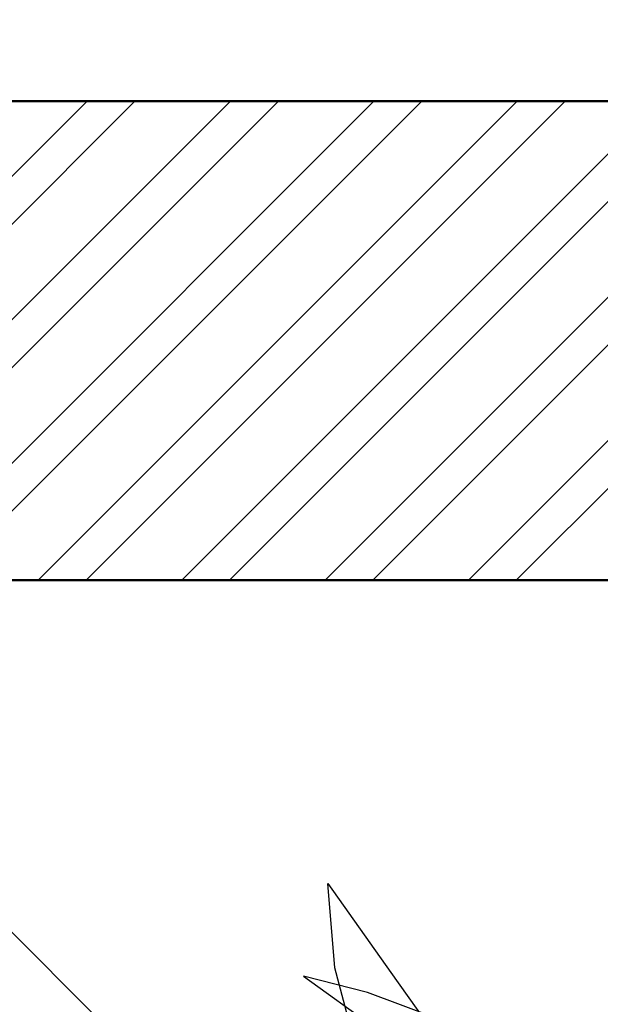
# Model space of a CAD drawing. Units: inches. Extents: x 3590 to 5167, y 65 to 1917.
# Tile 95 of 100: x 5034.93 to 5045.84, y 1789.03 to 1807.53. Entities that reach past the tile are written whole.
import ezdxf

# ---------------------------------------------------------------- set-up
doc = ezdxf.new("R2010")
doc.units = ezdxf.units.IN
for name, color, linetype, lineweight in [('A-ANNO-DIMS', 2, 'Continuous', 18), ('A-FLOR-PATT', 8, 'Continuous', 13), ('A-WALL', 7, 'Continuous', 50), ('A-WALL-PATT', 251, 'Continuous', 13), ('L-PLNT', 94, 'Continuous', 18)]:
    doc.layers.add(name, color=color, linetype=linetype, lineweight=lineweight)
doc.layers.add('DIENHOA', color=3, linetype='Continuous')
doc.styles.get("Standard").update_dxf_attribs({"font": 'arial.ttf'})
doc.dimstyles.new('ISO-25', dxfattribs={"dimtxt": 9, "dimasz": 2.5, "dimexe": 1.25, "dimexo": 0.625, "dimtad": 1, "dimdec": 1, "dimlunit": 3, "dimtxsty": 'Standard', "dimcen": 2.5, "dimadec": 0, "dimazin": 0, "dimtfac": 1, "dimtdec": 1, "dimtmove": 0, "dimatfit": 3, "dimfxl": 1, "dimarcsym": 0})

# ---------------------------------------------------------------- blocks, each defined once
blk = doc.blocks.new('*D101')
at = {"layer": 'A-ANNO-DIMS', "color": 0, "lineweight": -2, "transparency": 16777216}
for p, q in [((4420.274, 1806.624), (4420.274, 1818.615)), ((5080.274, 1806.624), (5080.274, 1818.615)), ((4422.774, 1817.365), (5077.774, 1817.365))]:
    blk.add_line(p, q, dxfattribs=at)
at = {"layer": 'A-ANNO-DIMS', "color": 0, "transparency": 16777216}
for points in [[(4422.774, 1817.781), (4422.774, 1816.948), (4420.274, 1817.365)], [(5077.774, 1817.781), (5077.774, 1816.948), (5080.274, 1817.365)]]:
    blk.add_solid(points, dxfattribs=at)
at = {"layer": 'Defpoints', "color": 0, "transparency": 16777216}
for p in [(5080.274, 1817.365), (4420.274, 1805.999), (5080.274, 1805.999)]:
    blk.add_point(p, dxfattribs=at)
at = {"layer": 'A-ANNO-DIMS', "color": 0, "transparency": 16777216, "insert": (4750.274, 1822.566), "char_height": 9, "attachment_point": 5}
blk.add_mtext("55'", dxfattribs=at)
blk = doc.blocks.new('Cay03_mb')
at = {"layer": 'DIENHOA'}
for p, q in [((-365.2, 390.27), (-414.37, 402.78)), ((-414.37, 402.78), (-240.22, 277.83)), ((-314.87, 371.26), (-365.2, 390.27))]:
    blk.add_line(p, q, dxfattribs=at)
for points in [[(-395.6, 473.65), (-347.51, 405.62), (-300.58, 339.5), (-254.33, 275.13), (-208.27, 212.32), (-161.92, 150.91), (-114.81, 90.72), (-66.46, 31.56), (-16.39, -26.73)], [(-16.39, -26.73), (-108.35, 38.55), (-186.88, 101.73), (-252.35, 163.45), (-305.09, 224.39), (-345.44, 285.22), (-373.75, 346.59), (-390.35, 409.18), (-395.6, 473.65)]]:
    blk.add_lwpolyline(points, dxfattribs=at)
blk = doc.blocks.new('*D323')
at = {"layer": 'A-ANNO-DIMS', "color": 0, "lineweight": -2, "transparency": 16777216}
for p, q in [((5069.172, 1795.216), (5069.172, 1874.95)), ((5065.437, 1795.216), (5070.422, 1795.216)), ((5069.172, 1769.309), (5069.172, 1792.716)), ((5065.437, 1766.809), (5070.422, 1766.809))]:
    blk.add_line(p, q, dxfattribs=at)
at = {"layer": 'A-ANNO-DIMS', "color": 0, "transparency": 16777216}
for points in [[(5068.756, 1792.716), (5069.589, 1792.716), (5069.172, 1795.216)], [(5068.756, 1769.309), (5069.589, 1769.309), (5069.172, 1766.809)]]:
    blk.add_solid(points, dxfattribs=at)
at = {"layer": 'Defpoints', "color": 0, "transparency": 16777216}
for p in [(5064.812, 1795.216), (5069.172, 1795.216), (5064.812, 1766.809)]:
    blk.add_point(p, dxfattribs=at)
at = {"layer": 'A-ANNO-DIMS', "color": 0, "transparency": 16777216, "insert": (5063.894, 1836.333), "char_height": 9, "attachment_point": 5, "rotation": 90}
blk.add_mtext('2\'-4 1/2" TYP.', dxfattribs=at)

msp = doc.modelspace()

# ---------------------------------------------------------------- hatches: boundary and pattern name
at = {"layer": 'A-FLOR-PATT', "transparency": 33554687}
h = msp.add_hatch(dxfattribs=at)
h.set_pattern_fill('AR-HBONE', color=256, scale=0.2)
h.set_pattern_definition([(45, (-588.972, 0), (0, 28.73682), [60.96, -20.32]), (135, (-574.604, 14.368), (3e-15, 28.73682), [60.96, -20.32])])
h.paths.add_polyline_path([(5071.274, 1796.999), (4933.274, 1796.999), (4933.274, 1753.999), (4962.774, 1753.999, -0.414214), (4928.774, 1719.999), (4933.274, 1718.999), (4933.274, 1334.999), (5071.274, 1334.999)])
h.paths.add_polyline_path([(4951.78, 1521.077), (4951.715, 1521.04), (4951.563, 1520.895)], flags=16)
h.paths.add_polyline_path([(4952.267, 1521.376), (4952.198, 1521.371), (4952.198, 1521.356)], flags=0)
h.paths.add_polyline_path([(4967.051, 1529.728), (4965.231, 1528.694), (4963.411, 1527.714), (4961.756, 1526.851), (4963.589, 1527.449), (4964.036, 1527.478), (4962.975, 1527.249), (4961.76, 1526.852), (4959.792, 1525.834), (4958.005, 1524.895), (4956.24, 1523.93), (4954.504, 1522.919), (4954.129, 1522.682), (4953.361, 1521.997), (4953.366, 1521.998), (4953.605, 1522.064), (4955.106, 1522.761), (4956.921, 1523.434), (4958.678, 1523.915), (4960.358, 1524.2), (4961.945, 1524.286), (4964.171, 1524.108), (4965.958, 1523.309), (4963.863, 1522.976), (4965.187, 1522.499), (4963.366, 1522.497), (4961.545, 1522.487), (4959.764, 1522.461), (4958.304, 1522.419), (4957.974, 1522.388), (4956.307, 1522.232), (4954.718, 1522.071), (4953.251, 1521.899), (4953.525, 1521.623), (4954.331, 1521.379), (4956.243, 1521.23), (4958.039, 1520.93), (4959.684, 1520.483), (4961.16, 1519.896), (4963.107, 1518.8), (4964.393, 1517.325), (4962.973, 1517.726), (4964.558, 1516.661), (4965.407, 1515.708), (4963.507, 1516.322), (4961.68, 1517.005), (4959.935, 1517.745), (4958.282, 1518.528), (4956.732, 1519.343), (4955.295, 1520.175), (4954.672, 1520.572), (4954.513, 1520.627), (4955.658, 1519.318), (4956.703, 1517.982), (4957.644, 1516.647), (4958.485, 1515.334), (4959.55, 1513.524), (4960.438, 1511.769), (4958.841, 1513.62), (4957.452, 1515.325), (4955.819, 1517.459), (4956.665, 1515.448), (4957.111, 1513.923), (4957.447, 1511.714), (4957.076, 1509.793), (4956.538, 1511.11), (4955.992, 1512.569), (4955.444, 1514.125), (4954.898, 1515.735), (4954.357, 1517.356), (4953.824, 1518.943), (4953.305, 1520.452), (4953.065, 1521.116), (4952.971, 1521.146), (4952.949, 1521.086), (4952.73, 1520.199), (4953.37, 1518.024), (4953.757, 1516.373), (4954.051, 1514.765), (4954.264, 1513.221), (4954.471, 1511.131), (4954.497, 1510.402), (4954.409, 1511.76), (4954.264, 1513.221), (4954.051, 1514.765), (4953.757, 1516.373), (4953.37, 1518.024), (4952.877, 1519.698), (4952.716, 1520.141), (4952.533, 1519.059), (4952.374, 1517.789), (4952.219, 1516.312), (4952.046, 1514.6), (4951.833, 1512.626), (4951.557, 1510.363), (4951.203, 1512.168), (4950.852, 1514.339), (4950.985, 1516.376), (4951.66, 1518.286), (4952.593, 1520.481), (4952.357, 1521.13), (4951.855, 1520.328), (4950.839, 1518.908), (4949.777, 1517.587), (4948.916, 1516.617), (4948.111, 1515.256), (4947.089, 1513.554), (4945.889, 1511.615), (4946.326, 1513.402), (4946.562, 1514.249), (4945.528, 1513.327), (4944.581, 1512.531), (4946.018, 1514.508), (4947.204, 1516.048), (4947.893, 1517.313), (4949.307, 1518.764), (4950.414, 1519.767), (4950.451, 1519.806), (4952.267, 1521.376), (4951.645, 1521.493), (4950.404, 1521.18), (4948.044, 1520.359), (4946.119, 1519.452), (4944.572, 1518.475), (4943.35, 1517.443), (4941.997, 1515.92), (4941.661, 1515.275), (4942.813, 1516.99), (4944.572, 1518.475), (4946.119, 1519.452), (4948.044, 1520.359), (4950.404, 1521.18), (4951.645, 1521.493), (4949.647, 1521.868), (4948.6, 1521.756), (4947.126, 1521.57), (4945.42, 1521.348), (4943.45, 1521.105), (4941.183, 1520.856), (4942.86, 1521.613), (4943.873, 1522.03), (4942.952, 1521.909), (4941.41, 1521.485), (4939.543, 1520.67), (4938.968, 1520.226), (4940.733, 1521.299), (4942.952, 1521.909), (4943.702, 1522.008), (4945.894, 1522.7), (4947.565, 1522.714), (4948.921, 1522.566), (4951.131, 1522.183), (4950.971, 1522.297), (4948.129, 1523.006), (4946.035, 1523.707), (4944.232, 1524.521), (4942.707, 1525.461), (4941.444, 1526.537), (4940.43, 1527.761), (4939.649, 1529.143), (4941.421, 1528.122), (4943.147, 1527.132), (4944.841, 1526.175), (4946.514, 1525.25), (4948.179, 1524.359), (4948.365, 1524.263), (4946.475, 1526.045), (4945.181, 1527.54), (4944.19, 1529.033), (4943.496, 1530.54), (4943.278, 1531.36), (4942.498, 1531.919), (4943.114, 1531.762), (4942.959, 1533.659), (4944.14, 1531.989), (4944.612, 1531.323), (4946.202, 1530.463), (4947.486, 1529.509), (4948.79, 1528.226), (4950.368, 1526.237), (4949.485, 1528.155), (4948.851, 1530.123), (4948.491, 1532.041), (4948.381, 1533.918), (4948.501, 1535.76), (4948.827, 1537.573), (4949.418, 1535.565), (4949.957, 1533.569), (4950.464, 1531.586), (4950.961, 1529.617), (4951.391, 1527.954), (4951.724, 1530.687), (4952.201, 1532.58), (4952.889, 1534.33), (4953.77, 1535.951), (4954.827, 1537.46), (4954.521, 1535.39), (4954.273, 1533.937), (4955.58, 1535.663), (4956.748, 1536.739), (4956.159, 1534.78), (4955.589, 1532.873), (4955.043, 1531.006), (4954.525, 1529.166), (4954.038, 1527.341), (4953.638, 1525.733), (4953.611, 1525.586), (4953.398, 1524.166), (4953.382, 1524.009), (4954.07, 1525.476), (4954.912, 1527.022), (4956.136, 1528.894), (4957.847, 1530.577), (4959.376, 1531.54), (4958.256, 1530.104), (4957.143, 1528.663), (4956.066, 1527.243), (4955.056, 1525.871), (4954.141, 1524.571), (4953.352, 1523.372), (4953.311, 1523.303), (4953.273, 1522.925), (4953.261, 1522.382), (4954.103, 1523.373), (4954.63, 1524.284), (4955.961, 1526.358), (4957.23, 1528.13), (4958.421, 1529.609), (4960.037, 1531.368), (4961.374, 1532.375), (4962.101, 1532.77), (4961.07, 1531.061), (4959.987, 1529.438), (4958.869, 1527.908), (4958.15, 1527.007), (4959.803, 1528.003), (4961.589, 1528.793), (4963.391, 1529.328), (4965.211, 1529.632)], flags=16)
h.paths.add_polyline_path([(4962.944, 1523.182), (4961.107, 1523.422), (4960.392, 1523.362), (4962.35, 1523.331)], flags=0)
h.paths.add_polyline_path([(5049.541, 1584.551), (5049.476, 1584.515), (5049.325, 1584.37)], flags=16)
h.paths.add_polyline_path([(5050.028, 1584.851), (5049.959, 1584.845), (5049.959, 1584.83)], flags=0)
h.paths.add_polyline_path([(5042.333, 1581.949), (5043.88, 1582.926), (5045.806, 1583.833), (5048.165, 1584.654), (5049.406, 1584.967), (5047.408, 1585.342), (5046.361, 1585.231), (5044.888, 1585.044), (5043.181, 1584.822), (5041.211, 1584.579), (5038.944, 1584.33), (5040.622, 1585.087), (5041.634, 1585.504), (5040.713, 1585.383), (5039.171, 1584.959), (5037.304, 1584.144), (5036.729, 1583.7), (5038.494, 1584.773), (5040.713, 1585.383), (5041.463, 1585.482), (5043.655, 1586.174), (5045.326, 1586.188), (5046.682, 1586.04), (5048.893, 1585.657), (5048.732, 1585.771), (5045.891, 1586.48), (5043.796, 1587.181), (5041.994, 1587.996), (5040.468, 1588.935), (5039.205, 1590.011), (5038.191, 1591.235), (5037.41, 1592.617), (5039.182, 1591.596), (5040.909, 1590.607), (5042.602, 1589.649), (5044.275, 1588.724), (5045.94, 1587.833), (5046.126, 1587.738), (5044.237, 1589.519), (5042.942, 1591.015), (5041.952, 1592.508), (5041.257, 1594.014), (5041.039, 1594.834), (5040.26, 1595.393), (5040.875, 1595.237), (5040.721, 1597.133), (5041.901, 1595.463), (5042.373, 1594.798), (5043.963, 1593.938), (5045.247, 1592.983), (5046.552, 1591.701), (5048.129, 1589.712), (5047.247, 1591.63), (5046.613, 1593.597), (5046.252, 1595.515), (5046.142, 1597.392), (5046.262, 1599.234), (5046.588, 1601.047), (5047.179, 1599.039), (5047.718, 1597.043), (5048.225, 1595.06), (5048.722, 1593.091), (5049.152, 1591.429), (5049.485, 1594.161), (5049.962, 1596.054), (5050.65, 1597.804), (5051.532, 1599.425), (5052.589, 1600.934), (5052.283, 1598.864), (5052.034, 1597.411), (5053.341, 1599.137), (5054.509, 1600.213), (5053.92, 1598.254), (5053.35, 1596.348), (5052.805, 1594.48), (5052.286, 1592.64), (5051.799, 1590.815), (5051.4, 1589.207), (5051.373, 1589.06), (5051.159, 1587.64), (5051.143, 1587.483), (5051.831, 1588.95), (5052.673, 1590.496), (5053.898, 1592.368), (5055.608, 1594.051), (5057.137, 1595.014), (5056.017, 1593.578), (5054.904, 1592.137), (5053.828, 1590.717), (5052.817, 1589.345), (5051.902, 1588.046), (5051.113, 1586.846), (5051.072, 1586.777), (5051.034, 1586.399), (5051.022, 1585.856), (5051.864, 1586.847), (5052.391, 1587.758), (5053.723, 1589.832), (5054.991, 1591.604), (5056.182, 1593.083), (5057.798, 1594.842), (5059.135, 1595.849), (5059.863, 1596.244), (5058.831, 1594.535), (5057.749, 1592.912), (5056.63, 1591.382), (5055.912, 1590.482), (5057.564, 1591.477), (5059.35, 1592.267), (5061.152, 1592.802), (5062.972, 1593.106), (5064.812, 1593.203), (5062.992, 1592.169), (5061.172, 1591.188), (5059.518, 1590.325), (5061.35, 1590.924), (5061.797, 1590.952), (5060.737, 1590.723), (5059.521, 1590.326), (5057.553, 1589.308), (5055.766, 1588.369), (5054.002, 1587.404), (5052.265, 1586.393), (5051.891, 1586.156), (5051.122, 1585.471), (5051.127, 1585.472), (5051.366, 1585.538), (5052.867, 1586.235), (5054.682, 1586.908), (5056.439, 1587.389), (5058.12, 1587.675), (5059.706, 1587.76), (5061.933, 1587.583), (5063.719, 1586.783), (5061.624, 1586.45), (5062.949, 1585.973), (5061.127, 1585.971), (5059.307, 1585.961), (5057.525, 1585.935), (5056.065, 1585.893), (5055.735, 1585.862), (5054.068, 1585.707), (5052.479, 1585.546), (5051.012, 1585.373), (5051.286, 1585.097), (5052.092, 1584.853), (5054.004, 1584.704), (5055.8, 1584.404), (5057.446, 1583.958), (5058.921, 1583.37), (5060.868, 1582.274), (5062.154, 1580.799), (5060.734, 1581.2), (5062.32, 1580.135), (5063.168, 1579.182), (5061.269, 1579.796), (5059.441, 1580.479), (5057.696, 1581.219), (5056.043, 1582.003), (5054.493, 1582.817), (5053.057, 1583.649), (5052.433, 1584.047), (5052.274, 1584.101), (5053.42, 1582.793), (5054.464, 1581.457), (5055.405, 1580.121), (5056.247, 1578.809), (5057.311, 1576.998), (5058.199, 1575.244), (5056.602, 1577.094), (5055.213, 1578.799), (5053.58, 1580.933), (5054.427, 1578.922), (5054.872, 1577.397), (5055.208, 1575.189), (5054.838, 1573.267), (5054.299, 1574.584), (5053.754, 1576.043), (5053.206, 1577.599), (5052.659, 1579.209), (5052.118, 1580.83), (5051.585, 1582.417), (5051.066, 1583.927), (5050.826, 1584.59), (5050.733, 1584.62), (5050.711, 1584.561), (5050.491, 1583.673), (5051.131, 1581.498), (5051.518, 1579.847), (5051.813, 1578.24), (5052.026, 1576.695), (5052.233, 1574.605), (5052.258, 1573.876), (5052.17, 1575.234), (5052.026, 1576.695), (5051.813, 1578.24), (5051.518, 1579.847), (5051.131, 1581.498), (5050.638, 1583.172), (5050.477, 1583.615), (5050.294, 1582.533), (5050.136, 1581.263), (5049.981, 1579.786), (5049.807, 1578.074), (5049.594, 1576.1), (5049.318, 1573.837), (5048.965, 1575.642), (5048.613, 1577.813), (5048.747, 1579.85), (5049.421, 1581.76), (5050.354, 1583.955), (5050.118, 1584.604), (5049.616, 1583.802), (5048.6, 1582.382), (5047.538, 1581.061), (5046.677, 1580.091), (5045.872, 1578.73), (5044.85, 1577.028), (5043.651, 1575.089), (5044.087, 1576.877), (5044.324, 1577.723), (5043.289, 1576.801), (5042.342, 1576.005), (5043.779, 1577.982), (5044.966, 1579.522), (5045.655, 1580.787), (5047.068, 1582.239), (5048.175, 1583.241), (5048.213, 1583.28), (5050.028, 1584.851), (5049.406, 1584.967), (5048.165, 1584.654), (5045.806, 1583.833), (5043.88, 1582.926), (5042.333, 1581.949), (5041.111, 1580.917), (5039.758, 1579.394), (5039.423, 1578.749), (5040.575, 1580.464)], flags=16)
h.paths.add_polyline_path([(4954.799, 1533.12), (4954.262, 1532.079), (4953.831, 1530.935), (4953.505, 1529.636), (4953.283, 1528.133), (4953.167, 1526.376), (4953.156, 1524.315), (4953.277, 1521.236), (4952.802, 1521.842), (4951.557, 1521.998), (4950.976, 1521.961), (4952.661, 1521.941), (4952.802, 1521.842), (4953.152, 1523.593), (4953.167, 1526.376), (4953.283, 1528.133), (4953.609, 1530.346), (4954.456, 1532.592)], flags=0)
h.paths.add_polyline_path([(5050.563, 1585.316), (5049.318, 1585.472), (5048.737, 1585.435), (5050.422, 1585.415), (5050.563, 1585.316), (5050.914, 1587.067), (5050.928, 1589.851), (5051.045, 1591.607), (5051.371, 1593.82), (5052.217, 1596.066), (5052.56, 1596.594), (5052.024, 1595.554), (5051.592, 1594.409), (5051.266, 1593.11), (5051.045, 1591.607), (5050.928, 1589.851), (5050.918, 1587.789), (5051.038, 1584.71)], flags=0)
h.paths.add_polyline_path([(5058.153, 1586.836), (5060.111, 1586.805), (5060.705, 1586.656), (5058.868, 1586.896)], flags=0)
h.paths.add_polyline_path([(5049.541, 1430.936), (5049.476, 1430.9), (5049.325, 1430.755)], flags=16)
h.paths.add_polyline_path([(5050.028, 1431.236), (5049.959, 1431.231), (5049.959, 1431.215)], flags=0)
h.paths.add_polyline_path([(5046.588, 1447.432), (5047.179, 1445.425), (5047.718, 1443.429), (5048.225, 1441.446), (5048.722, 1439.476), (5049.152, 1437.814), (5049.485, 1440.546), (5049.962, 1442.439), (5050.65, 1444.189), (5051.532, 1445.811), (5052.589, 1447.319), (5052.283, 1445.249), (5052.034, 1443.796), (5053.341, 1445.522), (5054.509, 1446.598), (5053.92, 1444.64), (5053.35, 1442.733), (5052.805, 1440.865), (5052.286, 1439.025), (5051.799, 1437.201), (5051.4, 1435.592), (5051.373, 1435.445), (5051.159, 1434.025), (5051.143, 1433.868), (5051.831, 1435.335), (5052.673, 1436.881), (5053.898, 1438.753), (5055.608, 1440.436), (5057.137, 1441.4), (5056.017, 1439.963), (5054.904, 1438.522), (5053.828, 1437.102), (5052.817, 1435.73), (5051.902, 1434.431), (5051.113, 1433.231), (5051.072, 1433.162), (5051.034, 1432.784), (5051.022, 1432.242), (5051.864, 1433.232), (5052.391, 1434.143), (5053.723, 1436.217), (5054.991, 1437.989), (5056.182, 1439.468), (5057.798, 1441.227), (5059.135, 1442.235), (5059.863, 1442.629), (5058.831, 1440.921), (5057.749, 1439.298), (5056.63, 1437.767), (5055.912, 1436.867), (5057.564, 1437.863), (5059.35, 1438.652), (5061.152, 1439.187), (5062.972, 1439.491), (5064.812, 1439.588), (5062.992, 1438.554), (5061.172, 1437.573), (5059.518, 1436.71), (5061.35, 1437.309), (5061.797, 1437.337), (5060.737, 1437.108), (5059.521, 1436.711), (5057.553, 1435.693), (5055.766, 1434.754), (5054.002, 1433.789), (5052.265, 1432.778), (5051.891, 1432.541), (5051.122, 1431.856), (5051.127, 1431.857), (5051.366, 1431.923), (5052.867, 1432.62), (5054.682, 1433.293), (5056.439, 1433.775), (5058.12, 1434.06), (5059.706, 1434.145), (5061.933, 1433.968), (5063.719, 1433.168), (5061.624, 1432.835), (5062.949, 1432.358), (5061.127, 1432.357), (5059.307, 1432.346), (5057.525, 1432.32), (5056.065, 1432.278), (5055.735, 1432.248), (5054.068, 1432.092), (5052.479, 1431.931), (5051.012, 1431.759), (5051.286, 1431.482), (5052.092, 1431.238), (5054.004, 1431.089), (5055.8, 1430.789), (5057.446, 1430.343), (5058.921, 1429.755), (5060.868, 1428.66), (5062.154, 1427.185), (5060.734, 1427.585), (5062.32, 1426.52), (5063.168, 1425.567), (5061.269, 1426.181), (5059.441, 1426.865), (5057.696, 1427.604), (5056.043, 1428.388), (5054.493, 1429.202), (5053.057, 1430.034), (5052.433, 1430.432), (5052.274, 1430.487), (5053.42, 1429.178), (5054.464, 1427.842), (5055.405, 1426.506), (5056.247, 1425.194), (5057.311, 1423.383), (5058.199, 1421.629), (5056.602, 1423.479), (5055.213, 1425.184), (5053.58, 1427.318), (5054.427, 1425.307), (5054.872, 1423.782), (5055.208, 1421.574), (5054.838, 1419.652), (5054.299, 1420.97), (5053.754, 1422.428), (5053.206, 1423.984), (5052.659, 1425.595), (5052.118, 1427.215), (5051.585, 1428.802), (5051.066, 1430.312), (5050.826, 1430.975), (5050.733, 1431.005), (5050.711, 1430.946), (5050.491, 1430.058), (5051.131, 1427.883), (5051.518, 1426.232), (5051.813, 1424.625), (5052.026, 1423.081), (5052.233, 1420.991), (5052.258, 1420.261), (5052.17, 1421.619), (5052.026, 1423.081), (5051.813, 1424.625), (5051.518, 1426.232), (5051.131, 1427.883), (5050.638, 1429.558), (5050.477, 1430.001), (5050.294, 1428.918), (5050.136, 1427.648), (5049.981, 1426.171), (5049.807, 1424.459), (5049.594, 1422.485), (5049.318, 1420.222), (5048.965, 1422.028), (5048.613, 1424.199), (5048.747, 1426.235), (5049.421, 1428.146), (5050.354, 1430.34), (5050.118, 1430.989), (5049.616, 1430.187), (5048.6, 1428.768), (5047.538, 1427.446), (5046.677, 1426.477), (5045.872, 1425.116), (5044.85, 1423.413), (5043.651, 1421.474), (5044.087, 1423.262), (5044.324, 1424.109), (5043.289, 1423.186), (5042.342, 1422.391), (5043.779, 1424.368), (5044.966, 1425.907), (5045.655, 1427.173), (5047.068, 1428.624), (5048.175, 1429.627), (5048.213, 1429.666), (5050.028, 1431.236), (5049.406, 1431.353), (5048.165, 1431.039), (5045.806, 1430.218), (5043.88, 1429.311), (5042.333, 1428.334), (5041.111, 1427.302), (5039.758, 1425.779), (5039.423, 1425.134), (5040.575, 1426.849), (5042.333, 1428.334), (5043.88, 1429.311), (5045.806, 1430.218), (5048.165, 1431.039), (5049.406, 1431.353), (5047.408, 1431.727), (5046.361, 1431.616), (5044.888, 1431.429), (5043.181, 1431.207), (5041.211, 1430.964), (5038.944, 1430.715), (5040.622, 1431.472), (5041.634, 1431.89), (5040.713, 1431.769), (5039.171, 1431.345), (5037.304, 1430.53), (5036.729, 1430.085), (5038.494, 1431.158), (5040.713, 1431.769), (5041.463, 1431.867), (5043.655, 1432.559), (5045.326, 1432.573), (5046.682, 1432.425), (5048.893, 1432.042), (5048.732, 1432.156), (5045.891, 1432.865), (5043.796, 1433.566), (5041.994, 1434.381), (5040.468, 1435.321), (5039.205, 1436.396), (5038.191, 1437.62), (5037.41, 1439.002), (5039.182, 1437.982), (5040.909, 1436.992), (5042.602, 1436.034), (5044.275, 1435.109), (5045.94, 1434.218), (5046.126, 1434.123), (5044.237, 1435.904), (5042.942, 1437.4), (5041.952, 1438.893), (5041.257, 1440.399), (5041.039, 1441.219), (5040.26, 1441.778), (5040.875, 1441.622), (5040.721, 1443.518), (5041.901, 1441.848), (5042.373, 1441.183), (5043.963, 1440.323), (5045.247, 1439.369), (5046.552, 1438.086), (5048.129, 1436.097), (5047.247, 1438.015), (5046.613, 1439.982), (5046.252, 1441.901), (5046.142, 1443.778), (5046.262, 1445.619)], flags=16)
h.paths.add_polyline_path([(5052.382, 1444.255), (5051.623, 1442.78), (5052.024, 1441.939), (5052.56, 1442.98)], flags=0)
h.paths.add_polyline_path([(5050.563, 1431.701), (5049.318, 1431.857), (5048.737, 1431.821), (5050.422, 1431.8)], flags=0)
h.paths.add_polyline_path([(5058.153, 1433.221), (5060.111, 1433.19), (5060.705, 1433.041), (5058.868, 1433.281)], flags=0)
h.paths.add_polyline_path([(5049.541, 1352.285), (5049.476, 1352.249), (5049.325, 1352.104)], flags=16)
h.paths.add_polyline_path([(5050.028, 1352.585), (5049.959, 1352.58), (5049.959, 1352.564)], flags=0)
h.paths.add_polyline_path([(5046.588, 1368.781), (5047.179, 1366.774), (5047.718, 1364.778), (5048.225, 1362.795), (5048.722, 1360.825), (5049.152, 1359.163), (5049.485, 1361.896), (5049.962, 1363.789), (5050.65, 1365.538), (5051.532, 1367.16), (5052.589, 1368.669), (5052.283, 1366.598), (5052.034, 1365.145), (5053.341, 1366.871), (5054.509, 1367.947), (5053.92, 1365.989), (5053.35, 1364.082), (5052.805, 1362.214), (5052.286, 1360.374), (5051.799, 1358.55), (5051.4, 1356.942), (5051.373, 1356.794), (5051.159, 1355.374), (5051.143, 1355.218), (5051.831, 1356.684), (5052.673, 1358.23), (5053.898, 1360.102), (5055.608, 1361.786), (5057.137, 1362.749), (5056.017, 1361.313), (5054.904, 1359.872), (5053.828, 1358.452), (5052.817, 1357.079), (5051.902, 1355.78), (5051.113, 1354.581), (5051.072, 1354.512), (5051.034, 1354.133), (5051.022, 1353.591), (5051.864, 1354.581), (5052.391, 1355.492), (5053.723, 1357.566), (5054.991, 1359.338), (5056.182, 1360.817), (5057.798, 1362.577), (5059.135, 1363.584), (5059.863, 1363.979), (5058.831, 1362.27), (5057.749, 1360.647), (5056.63, 1359.117), (5055.912, 1358.216), (5057.564, 1359.212), (5059.35, 1360.001), (5061.152, 1360.536), (5062.972, 1360.841), (5064.812, 1360.937), (5062.992, 1359.903), (5061.172, 1358.923), (5059.518, 1358.059), (5061.35, 1358.658), (5061.797, 1358.687), (5060.737, 1358.458), (5059.521, 1358.061), (5057.553, 1357.043), (5055.766, 1356.103), (5054.002, 1355.138), (5052.265, 1354.127), (5051.891, 1353.89), (5051.122, 1353.206), (5051.127, 1353.206), (5051.366, 1353.272), (5052.867, 1353.969), (5054.682, 1354.643), (5056.439, 1355.124), (5058.12, 1355.409), (5059.706, 1355.495), (5061.933, 1355.317), (5063.719, 1354.518), (5061.624, 1354.184), (5062.949, 1353.708), (5061.127, 1353.706), (5059.307, 1353.695), (5057.525, 1353.669), (5056.065, 1353.627), (5055.735, 1353.597), (5054.068, 1353.441), (5052.479, 1353.28), (5051.012, 1353.108), (5051.286, 1352.831), (5052.092, 1352.587), (5054.004, 1352.439), (5055.8, 1352.138), (5057.446, 1351.692), (5058.921, 1351.104), (5060.868, 1350.009), (5062.154, 1348.534), (5060.734, 1348.935), (5062.32, 1347.869), (5063.168, 1346.916), (5061.269, 1347.53), (5059.441, 1348.214), (5057.696, 1348.954), (5056.043, 1349.737), (5054.493, 1350.551), (5053.057, 1351.383), (5052.433, 1351.781), (5052.274, 1351.836), (5053.42, 1350.527), (5054.464, 1349.191), (5055.405, 1347.855), (5056.247, 1346.543), (5057.311, 1344.733), (5058.199, 1342.978), (5056.602, 1344.828), (5055.213, 1346.534), (5053.58, 1348.667), (5054.427, 1346.656), (5054.872, 1345.132), (5055.208, 1342.923), (5054.838, 1341.002), (5054.299, 1342.319), (5053.754, 1343.778), (5053.206, 1345.334), (5052.659, 1346.944), (5052.118, 1348.564), (5051.585, 1350.151), (5051.066, 1351.661), (5050.826, 1352.324), (5050.733, 1352.355), (5050.711, 1352.295), (5050.491, 1351.408), (5051.131, 1349.232), (5051.518, 1347.581), (5051.813, 1345.974), (5052.026, 1344.43), (5052.233, 1342.34), (5052.258, 1341.61), (5052.17, 1342.969), (5052.026, 1344.43), (5051.813, 1345.974), (5051.518, 1347.581), (5051.131, 1349.232), (5050.638, 1350.907), (5050.477, 1351.35), (5050.294, 1350.267), (5050.136, 1348.997), (5049.981, 1347.52), (5049.807, 1345.809), (5049.594, 1343.835), (5049.318, 1341.571), (5048.965, 1343.377), (5048.613, 1345.548), (5048.747, 1347.585), (5049.421, 1349.495), (5050.354, 1351.689), (5050.118, 1352.339), (5049.616, 1351.536), (5048.6, 1350.117), (5047.538, 1348.795), (5046.677, 1347.826), (5045.872, 1346.465), (5044.85, 1344.763), (5043.651, 1342.824), (5044.087, 1344.611), (5044.324, 1345.458), (5043.289, 1344.535), (5042.342, 1343.74), (5043.779, 1345.717), (5044.966, 1347.256), (5045.655, 1348.522), (5047.068, 1349.973), (5048.175, 1350.976), (5048.213, 1351.015), (5050.028, 1352.585), (5049.406, 1352.702), (5048.165, 1352.388), (5045.806, 1351.567), (5043.88, 1350.661), (5042.333, 1349.683), (5041.111, 1348.651), (5039.758, 1347.128), (5039.423, 1346.483), (5040.575, 1348.198), (5042.333, 1349.683), (5043.88, 1350.661), (5045.806, 1351.567), (5048.165, 1352.388), (5049.406, 1352.702), (5047.408, 1353.076), (5046.361, 1352.965), (5044.888, 1352.779), (5043.181, 1352.556), (5041.211, 1352.313), (5038.944, 1352.065), (5040.622, 1352.821), (5041.634, 1353.239), (5040.713, 1353.118), (5039.171, 1352.694), (5037.304, 1351.879), (5036.729, 1351.434), (5038.494, 1352.508), (5040.713, 1353.118), (5041.463, 1353.216), (5043.655, 1353.909), (5045.326, 1353.923), (5046.682, 1353.774), (5048.893, 1353.391), (5048.732, 1353.506), (5045.891, 1354.214), (5043.796, 1354.915), (5041.994, 1355.73), (5040.468, 1356.67), (5039.205, 1357.746), (5038.191, 1358.969), (5037.41, 1360.352), (5039.182, 1359.331), (5040.909, 1358.341), (5042.602, 1357.383), (5044.275, 1356.458), (5045.94, 1355.567), (5046.126, 1355.472), (5044.237, 1357.253), (5042.942, 1358.749), (5041.952, 1360.242), (5041.257, 1361.748), (5041.039, 1362.568), (5040.26, 1363.128), (5040.875, 1362.971), (5040.721, 1364.867), (5041.901, 1363.197), (5042.373, 1362.532), (5043.963, 1361.672), (5045.247, 1360.718), (5046.552, 1359.435), (5048.129, 1357.446), (5047.247, 1359.364), (5046.613, 1361.331), (5046.252, 1363.25), (5046.142, 1365.127), (5046.262, 1366.969)], flags=16)
h.paths.add_polyline_path([(5052.382, 1365.604), (5051.623, 1364.129), (5052.024, 1363.288), (5052.56, 1364.329)], flags=0)
h.paths.add_polyline_path([(4951.78, 1698.041), (4951.715, 1698.005), (4951.563, 1697.859)], flags=16)
h.paths.add_polyline_path([(4952.267, 1698.341), (4952.198, 1698.335), (4952.198, 1698.32)], flags=0)
h.paths.add_polyline_path([(4957.076, 1686.757), (4956.538, 1688.074), (4955.992, 1689.533), (4955.444, 1691.089), (4954.898, 1692.699), (4954.357, 1694.32), (4953.824, 1695.907), (4953.305, 1697.417), (4953.065, 1698.08), (4952.971, 1698.11), (4952.949, 1698.051), (4952.73, 1697.163), (4953.37, 1694.988), (4953.757, 1693.337), (4954.051, 1691.729), (4954.264, 1690.185), (4954.471, 1688.095), (4954.497, 1687.366), (4954.409, 1688.724), (4954.264, 1690.185), (4954.051, 1691.729), (4953.757, 1693.337), (4953.37, 1694.988), (4952.877, 1696.662), (4952.716, 1697.105), (4952.533, 1696.023), (4952.374, 1694.753), (4952.219, 1693.276), (4952.046, 1691.564), (4951.833, 1689.59), (4951.557, 1687.327), (4951.203, 1689.132), (4950.852, 1691.303), (4950.985, 1693.34), (4951.66, 1695.25), (4952.593, 1697.445), (4952.357, 1698.094), (4951.855, 1697.292), (4950.839, 1695.872), (4949.777, 1694.551), (4948.916, 1693.581), (4948.111, 1692.22), (4947.089, 1690.518), (4945.889, 1688.579), (4946.326, 1690.366), (4946.562, 1691.213), (4945.528, 1690.291), (4944.581, 1689.495), (4946.018, 1691.472), (4947.204, 1693.012), (4947.893, 1694.277), (4949.307, 1695.729), (4950.414, 1696.731), (4950.451, 1696.77), (4952.267, 1698.341), (4951.645, 1698.457), (4950.404, 1698.144), (4948.044, 1697.323), (4946.119, 1696.416), (4944.572, 1695.439), (4943.35, 1694.407), (4941.997, 1692.884), (4941.661, 1692.239), (4942.813, 1693.954), (4944.572, 1695.439), (4946.119, 1696.416), (4948.044, 1697.323), (4950.404, 1698.144), (4951.645, 1698.457), (4949.647, 1698.832), (4948.6, 1698.72), (4947.126, 1698.534), (4945.42, 1698.312), (4943.45, 1698.069), (4941.183, 1697.82), (4942.86, 1698.577), (4943.873, 1698.994), (4942.952, 1698.873), (4941.41, 1698.449), (4939.543, 1697.634), (4938.968, 1697.19), (4940.733, 1698.263), (4942.952, 1698.873), (4943.702, 1698.972), (4945.894, 1699.664), (4947.565, 1699.678), (4948.921, 1699.53), (4951.131, 1699.147), (4950.971, 1699.261), (4948.129, 1699.97), (4946.035, 1700.671), (4944.232, 1701.486), (4942.707, 1702.425), (4941.444, 1703.501), (4940.43, 1704.725), (4939.649, 1706.107), (4941.421, 1705.086), (4943.147, 1704.097), (4944.841, 1703.139), (4946.514, 1702.214), (4948.179, 1701.323), (4948.365, 1701.227), (4946.475, 1703.009), (4945.181, 1704.505), (4944.19, 1705.997), (4943.496, 1707.504), (4943.278, 1708.324), (4942.498, 1708.883), (4943.114, 1708.727), (4942.959, 1710.623), (4944.14, 1708.953), (4944.612, 1708.287), (4946.202, 1707.428), (4947.486, 1706.473), (4948.79, 1705.191), (4950.368, 1703.202), (4949.485, 1705.12), (4948.851, 1707.087), (4948.491, 1709.005), (4948.381, 1710.882), (4948.501, 1712.724), (4948.827, 1714.537), (4949.418, 1712.529), (4949.957, 1710.533), (4950.464, 1708.55), (4950.961, 1706.581), (4951.391, 1704.919), (4951.724, 1707.651), (4952.201, 1709.544), (4952.889, 1711.294), (4953.77, 1712.915), (4954.827, 1714.424), (4954.521, 1712.354), (4954.273, 1710.901), (4955.58, 1712.627), (4956.748, 1713.703), (4956.159, 1711.744), (4955.589, 1709.837), (4955.043, 1707.97), (4954.525, 1706.13), (4954.038, 1704.305), (4953.638, 1702.697), (4953.611, 1702.55), (4953.398, 1701.13), (4953.382, 1700.973), (4954.07, 1702.44), (4954.912, 1703.986), (4956.136, 1705.858), (4957.847, 1707.541), (4959.376, 1708.504), (4958.256, 1707.068), (4957.143, 1705.627), (4956.066, 1704.207), (4955.056, 1702.835), (4954.141, 1701.536), (4953.352, 1700.336), (4953.311, 1700.267), (4953.273, 1699.889), (4953.261, 1699.346), (4954.103, 1700.337), (4954.63, 1701.248), (4955.961, 1703.322), (4957.23, 1705.094), (4958.421, 1706.573), (4960.037, 1708.332), (4961.374, 1709.339), (4962.101, 1709.734), (4961.07, 1708.025), (4959.987, 1706.402), (4958.869, 1704.872), (4958.15, 1703.972), (4959.803, 1704.967), (4961.589, 1705.757), (4963.391, 1706.292), (4965.211, 1706.596), (4967.051, 1706.692), (4965.231, 1705.659), (4963.411, 1704.678), (4961.756, 1703.815), (4963.589, 1704.413), (4964.036, 1704.442), (4962.975, 1704.213), (4961.76, 1703.816), (4959.792, 1702.798), (4958.005, 1701.859), (4956.24, 1700.894), (4954.504, 1699.883), (4954.129, 1699.646), (4953.361, 1698.961), (4953.366, 1698.962), (4953.605, 1699.028), (4955.106, 1699.725), (4956.921, 1700.398), (4958.678, 1700.879), (4960.358, 1701.164), (4961.945, 1701.25), (4964.171, 1701.073), (4965.958, 1700.273), (4963.863, 1699.94), (4965.187, 1699.463), (4963.366, 1699.461), (4961.545, 1699.451), (4959.764, 1699.425), (4958.304, 1699.383), (4957.974, 1699.352), (4956.307, 1699.197), (4954.718, 1699.036), (4953.251, 1698.863), (4953.525, 1698.587), (4954.331, 1698.343), (4956.243, 1698.194), (4958.039, 1697.894), (4959.684, 1697.447), (4961.16, 1696.86), (4963.107, 1695.764), (4964.393, 1694.289), (4962.973, 1694.69), (4964.558, 1693.625), (4965.407, 1692.672), (4963.507, 1693.286), (4961.68, 1693.969), (4959.935, 1694.709), (4958.282, 1695.492), (4956.732, 1696.307), (4955.295, 1697.139), (4954.672, 1697.536), (4954.513, 1697.591), (4955.658, 1696.282), (4956.703, 1694.946), (4957.644, 1693.611), (4958.485, 1692.298), (4959.55, 1690.488), (4960.438, 1688.733), (4958.841, 1690.584), (4957.452, 1692.289), (4955.819, 1694.423), (4956.665, 1692.412), (4957.111, 1690.887), (4957.447, 1688.678)], flags=16)
h.paths.add_polyline_path([(5050.563, 1353.05), (5049.318, 1353.207), (5048.737, 1353.17), (5050.422, 1353.15)], flags=0)
h.paths.add_polyline_path([(4951.78, 1351.486), (4951.715, 1351.45), (4951.563, 1351.305)], flags=16)
h.paths.add_polyline_path([(4952.267, 1351.786), (4952.198, 1351.78), (4952.198, 1351.765)], flags=0)
h.paths.add_polyline_path([(4954.827, 1367.869), (4954.521, 1365.799), (4954.273, 1364.346), (4955.58, 1366.072), (4956.748, 1367.148), (4956.159, 1365.19), (4955.589, 1363.283), (4955.043, 1361.415), (4954.525, 1359.575), (4954.038, 1357.751), (4953.638, 1356.142), (4953.611, 1355.995), (4953.398, 1354.575), (4953.382, 1354.418), (4954.07, 1355.885), (4954.912, 1357.431), (4956.136, 1359.303), (4957.847, 1360.986), (4959.376, 1361.95), (4958.256, 1360.513), (4957.143, 1359.072), (4956.066, 1357.652), (4955.056, 1356.28), (4954.141, 1354.981), (4953.352, 1353.781), (4953.311, 1353.712), (4953.273, 1353.334), (4953.261, 1352.792), (4954.103, 1353.782), (4954.63, 1354.693), (4955.961, 1356.767), (4957.23, 1358.539), (4958.421, 1360.018), (4960.037, 1361.777), (4961.374, 1362.785), (4962.101, 1363.179), (4961.07, 1361.471), (4959.987, 1359.848), (4958.869, 1358.317), (4958.15, 1357.417), (4959.803, 1358.413), (4961.589, 1359.202), (4963.391, 1359.737), (4965.211, 1360.041), (4967.051, 1360.138), (4965.231, 1359.104), (4963.411, 1358.123), (4961.756, 1357.26), (4963.589, 1357.859), (4964.036, 1357.887), (4962.975, 1357.658), (4961.76, 1357.261), (4959.792, 1356.243), (4958.005, 1355.304), (4956.24, 1354.339), (4954.504, 1353.328), (4954.129, 1353.091), (4953.361, 1352.406), (4953.366, 1352.407), (4953.605, 1352.473), (4955.106, 1353.17), (4956.921, 1353.843), (4958.678, 1354.325), (4960.358, 1354.61), (4961.945, 1354.695), (4964.171, 1354.518), (4965.958, 1353.718), (4963.863, 1353.385), (4965.187, 1352.908), (4963.366, 1352.907), (4961.545, 1352.896), (4959.764, 1352.87), (4958.304, 1352.828), (4957.974, 1352.798), (4956.307, 1352.642), (4954.718, 1352.481), (4953.251, 1352.309), (4953.525, 1352.032), (4954.331, 1351.788), (4956.243, 1351.639), (4958.039, 1351.339), (4959.684, 1350.893), (4961.16, 1350.305), (4963.107, 1349.21), (4964.393, 1347.735), (4962.973, 1348.135), (4964.558, 1347.07), (4965.407, 1346.117), (4963.507, 1346.731), (4961.68, 1347.414), (4959.935, 1348.154), (4958.282, 1348.938), (4956.732, 1349.752), (4955.295, 1350.584), (4954.672, 1350.982), (4954.513, 1351.036), (4955.658, 1349.728), (4956.703, 1348.392), (4957.644, 1347.056), (4958.485, 1345.744), (4959.55, 1343.933), (4960.438, 1342.179), (4958.841, 1344.029), (4957.452, 1345.734), (4955.819, 1347.868), (4956.665, 1345.857), (4957.111, 1344.332), (4957.447, 1342.124), (4957.076, 1340.202), (4956.538, 1341.52), (4955.992, 1342.978), (4955.444, 1344.534), (4954.898, 1346.145), (4954.357, 1347.765), (4953.824, 1349.352), (4953.305, 1350.862), (4953.065, 1351.525), (4952.971, 1351.555), (4952.949, 1351.496), (4952.73, 1350.608), (4953.37, 1348.433), (4953.757, 1346.782), (4954.051, 1345.175), (4954.264, 1343.631), (4954.471, 1341.541), (4954.497, 1340.811), (4954.409, 1342.169), (4954.264, 1343.631), (4954.051, 1345.175), (4953.757, 1346.782), (4953.37, 1348.433), (4952.877, 1350.108), (4952.716, 1350.551), (4952.533, 1349.468), (4952.374, 1348.198), (4952.219, 1346.721), (4952.046, 1345.009), (4951.833, 1343.035), (4951.557, 1340.772), (4951.203, 1342.578), (4950.852, 1344.749), (4950.985, 1346.785), (4951.66, 1348.696), (4952.593, 1350.89), (4952.357, 1351.539), (4951.855, 1350.737), (4950.839, 1349.318), (4949.777, 1347.996), (4948.916, 1347.027), (4948.111, 1345.665), (4947.089, 1343.963), (4945.889, 1342.024), (4946.326, 1343.812), (4946.562, 1344.659), (4945.528, 1343.736), (4944.581, 1342.941), (4946.018, 1344.918), (4947.204, 1346.457), (4947.893, 1347.723), (4949.307, 1349.174), (4950.414, 1350.177), (4950.451, 1350.216), (4952.267, 1351.786), (4951.645, 1351.903), (4950.404, 1351.589), (4948.044, 1350.768), (4946.119, 1349.861), (4944.572, 1348.884), (4943.35, 1347.852), (4941.997, 1346.329), (4941.661, 1345.684), (4942.813, 1347.399), (4944.572, 1348.884), (4946.119, 1349.861), (4948.044, 1350.768), (4950.404, 1351.589), (4951.645, 1351.903), (4949.647, 1352.277), (4948.6, 1352.166), (4947.126, 1351.979), (4945.42, 1351.757), (4943.45, 1351.514), (4941.183, 1351.265), (4942.86, 1352.022), (4943.873, 1352.44), (4942.952, 1352.319), (4941.41, 1351.895), (4939.543, 1351.08), (4938.968, 1350.635), (4940.733, 1351.708), (4942.952, 1352.319), (4943.702, 1352.417), (4945.894, 1353.109), (4947.565, 1353.123), (4948.921, 1352.975), (4951.131, 1352.592), (4950.971, 1352.706), (4948.129, 1353.415), (4946.035, 1354.116), (4944.232, 1354.931), (4942.707, 1355.871), (4941.444, 1356.946), (4940.43, 1358.17), (4939.649, 1359.552), (4941.421, 1358.532), (4943.147, 1357.542), (4944.841, 1356.584), (4946.514, 1355.659), (4948.179, 1354.768), (4948.365, 1354.673), (4946.475, 1356.454), (4945.181, 1357.95), (4944.19, 1359.443), (4943.496, 1360.949), (4943.278, 1361.769), (4942.498, 1362.328), (4943.114, 1362.172), (4942.959, 1364.068), (4944.14, 1362.398), (4944.612, 1361.733), (4946.202, 1360.873), (4947.486, 1359.919), (4948.79, 1358.636), (4950.368, 1356.647), (4949.485, 1358.565), (4948.851, 1360.532), (4948.491, 1362.451), (4948.381, 1364.328), (4948.501, 1366.169), (4948.827, 1367.982), (4949.418, 1365.975), (4949.957, 1363.979), (4950.464, 1361.995), (4950.961, 1360.026), (4951.391, 1358.364), (4951.724, 1361.096), (4952.201, 1362.989), (4952.889, 1364.739), (4953.77, 1366.361)], flags=16)
h.paths.add_polyline_path([(4954.799, 1363.53), (4954.262, 1362.489), (4953.831, 1361.344), (4953.505, 1360.045), (4953.283, 1358.543), (4953.167, 1356.786), (4953.156, 1354.724), (4953.277, 1351.646), (4952.802, 1352.251), (4951.557, 1352.407), (4950.976, 1352.371), (4952.661, 1352.35), (4952.802, 1352.251), (4953.152, 1354.002), (4953.167, 1356.786), (4953.283, 1358.543), (4953.609, 1360.755), (4954.456, 1363.001)], flags=0)
h.paths.add_polyline_path([(4952.802, 1698.806), (4951.557, 1698.962), (4950.976, 1698.925), (4952.661, 1698.905), (4952.802, 1698.806), (4953.152, 1700.557), (4953.167, 1703.34), (4953.283, 1705.097), (4953.609, 1707.31), (4954.456, 1709.556), (4954.799, 1710.084), (4954.262, 1709.043), (4953.831, 1707.899), (4953.505, 1706.6), (4953.283, 1705.097), (4953.167, 1703.34), (4953.156, 1701.279), (4953.277, 1698.2)], flags=0)
h.paths.add_polyline_path([(4962.944, 1700.146), (4961.107, 1700.386), (4960.392, 1700.326), (4962.35, 1700.295)], flags=0)
h.paths.add_polyline_path([(5058.153, 1354.57), (5060.111, 1354.539), (5060.705, 1354.391), (5058.868, 1354.631)], flags=0)
h.paths.add_polyline_path([(4962.944, 1353.591), (4961.107, 1353.831), (4960.392, 1353.771), (4962.35, 1353.74)], flags=0)
h.paths.add_polyline_path([(5049.541, 1778.72), (5049.476, 1778.684), (5049.325, 1778.539)], flags=16)
h.paths.add_polyline_path([(5050.028, 1779.02), (5049.959, 1779.014), (5049.959, 1778.999)], flags=0)
h.paths.add_polyline_path([(5052.258, 1768.045), (5052.17, 1769.403), (5052.026, 1770.864), (5051.813, 1772.409), (5051.518, 1774.016), (5051.131, 1775.667), (5050.638, 1777.341), (5050.477, 1777.784), (5050.294, 1776.702), (5050.136, 1775.432), (5049.981, 1773.955), (5049.807, 1772.243), (5049.594, 1770.269), (5049.318, 1768.006), (5048.965, 1769.811), (5048.613, 1771.982), (5048.747, 1774.019), (5049.421, 1775.929), (5050.354, 1778.124), (5050.118, 1778.773), (5049.616, 1777.971), (5048.6, 1776.551), (5047.538, 1775.23), (5046.677, 1774.26), (5045.872, 1772.899), (5044.85, 1771.197), (5043.651, 1769.258), (5044.087, 1771.046), (5044.324, 1771.892), (5043.289, 1770.97), (5042.342, 1770.174), (5043.779, 1772.151), (5044.966, 1773.691), (5045.655, 1774.956), (5047.068, 1776.408), (5048.175, 1777.41), (5048.213, 1777.449), (5050.028, 1779.02), (5049.406, 1779.136), (5048.165, 1778.823), (5045.806, 1778.002), (5043.88, 1777.095), (5042.333, 1776.118), (5041.111, 1775.086), (5039.758, 1773.563), (5039.423, 1772.918), (5040.575, 1774.633), (5042.333, 1776.118), (5043.88, 1777.095), (5045.806, 1778.002), (5048.165, 1778.823), (5049.406, 1779.136), (5047.408, 1779.511), (5046.361, 1779.4), (5044.888, 1779.213), (5043.181, 1778.991), (5041.211, 1778.748), (5038.944, 1778.499), (5040.622, 1779.256), (5041.634, 1779.673), (5040.713, 1779.552), (5039.171, 1779.128), (5037.304, 1778.313), (5036.729, 1777.869), (5038.494, 1778.942), (5040.713, 1779.552), (5041.463, 1779.651), (5043.655, 1780.343), (5045.326, 1780.357), (5046.682, 1780.209), (5048.893, 1779.826), (5048.732, 1779.94), (5045.891, 1780.649), (5043.796, 1781.35), (5041.994, 1782.165), (5040.468, 1783.104), (5039.205, 1784.18), (5038.191, 1785.404), (5037.41, 1786.786), (5039.182, 1785.765), (5040.909, 1784.776), (5042.602, 1783.818), (5044.275, 1782.893), (5045.94, 1782.002), (5046.126, 1781.907), (5044.237, 1783.688), (5042.942, 1785.184), (5041.952, 1786.677), (5041.257, 1788.183), (5041.039, 1789.003), (5040.26, 1789.562), (5040.875, 1789.406), (5040.721, 1791.302), (5041.901, 1789.632), (5042.373, 1788.967), (5043.963, 1788.107), (5045.247, 1787.152), (5046.552, 1785.87), (5048.129, 1783.881), (5047.247, 1785.799), (5046.613, 1787.766), (5046.252, 1789.684), (5046.142, 1791.561), (5046.262, 1793.403), (5046.588, 1795.216), (5047.179, 1793.208), (5047.718, 1791.213), (5048.225, 1789.229), (5048.722, 1787.26), (5049.152, 1785.598), (5049.485, 1788.33), (5049.962, 1790.223), (5050.65, 1791.973), (5051.532, 1793.594), (5052.589, 1795.103), (5052.283, 1793.033), (5052.034, 1791.58), (5053.341, 1793.306), (5054.509, 1794.382), (5053.92, 1792.423), (5053.35, 1790.517), (5052.805, 1788.649), (5052.286, 1786.809), (5051.799, 1784.984), (5051.4, 1783.376), (5051.373, 1783.229), (5051.159, 1781.809), (5051.143, 1781.652), (5051.831, 1783.119), (5052.673, 1784.665), (5053.898, 1786.537), (5055.608, 1788.22), (5057.137, 1789.183), (5056.017, 1787.747), (5054.904, 1786.306), (5053.828, 1784.886), (5052.817, 1783.514), (5051.902, 1782.215), (5051.113, 1781.015), (5051.072, 1780.946), (5051.034, 1780.568), (5051.022, 1780.025), (5051.864, 1781.016), (5052.391, 1781.927), (5053.723, 1784.001), (5054.991, 1785.773), (5056.182, 1787.252), (5057.798, 1789.011), (5059.135, 1790.018), (5059.863, 1790.413), (5058.831, 1788.704), (5057.749, 1787.081), (5056.63, 1785.551), (5055.912, 1784.651), (5057.564, 1785.646), (5059.35, 1786.436), (5061.152, 1786.971), (5062.972, 1787.275), (5064.812, 1787.372), (5062.992, 1786.338), (5061.172, 1785.357), (5059.518, 1784.494), (5061.35, 1785.093), (5061.797, 1785.121), (5060.737, 1784.892), (5059.521, 1784.495), (5057.553, 1783.477), (5055.766, 1782.538), (5054.002, 1781.573), (5052.265, 1780.562), (5051.891, 1780.325), (5051.122, 1779.64), (5051.127, 1779.641), (5051.366, 1779.707), (5052.867, 1780.404), (5054.682, 1781.077), (5056.439, 1781.558), (5058.12, 1781.844), (5059.706, 1781.929), (5061.933, 1781.752), (5063.719, 1780.952), (5061.624, 1780.619), (5062.949, 1780.142), (5061.127, 1780.14), (5059.307, 1780.13), (5057.525, 1780.104), (5056.065, 1780.062), (5055.735, 1780.031), (5054.068, 1779.876), (5052.479, 1779.715), (5051.012, 1779.542), (5051.286, 1779.266), (5052.092, 1779.022), (5054.004, 1778.873), (5055.8, 1778.573), (5057.446, 1778.127), (5058.921, 1777.539), (5060.868, 1776.443), (5062.154, 1774.968), (5060.734, 1775.369), (5062.32, 1774.304), (5063.168, 1773.351), (5061.269, 1773.965), (5059.441, 1774.648), (5057.696, 1775.388), (5056.043, 1776.172), (5054.493, 1776.986), (5053.057, 1777.818), (5052.433, 1778.216), (5052.274, 1778.27), (5053.42, 1776.962), (5054.464, 1775.626), (5055.405, 1774.29), (5056.247, 1772.978), (5057.311, 1771.167), (5058.199, 1769.413), (5056.602, 1771.263), (5055.213, 1772.968), (5053.58, 1775.102), (5054.427, 1773.091), (5054.872, 1771.566), (5055.208, 1769.358), (5054.838, 1767.436), (5054.299, 1768.753), (5053.754, 1770.212), (5053.206, 1771.768), (5052.659, 1773.378), (5052.118, 1774.999), (5051.585, 1776.586), (5051.066, 1778.096), (5050.826, 1778.759), (5050.733, 1778.789), (5050.711, 1778.73), (5050.491, 1777.842), (5051.131, 1775.667), (5051.518, 1774.016), (5051.813, 1772.409), (5052.026, 1770.864), (5052.233, 1768.774)], flags=16)
h.paths.add_polyline_path([(5050.563, 1779.485), (5049.318, 1779.641), (5048.737, 1779.604), (5050.422, 1779.584), (5050.563, 1779.485), (5050.914, 1781.236), (5050.928, 1784.02), (5051.045, 1785.776), (5051.371, 1787.989), (5052.217, 1790.235), (5052.56, 1790.763), (5052.024, 1789.723), (5051.592, 1788.578), (5051.266, 1787.279), (5051.045, 1785.776), (5050.928, 1784.02), (5050.918, 1781.958), (5051.038, 1778.879)], flags=0)
h.paths.add_polyline_path([(5058.153, 1781.005), (5060.111, 1780.974), (5060.705, 1780.825), (5058.868, 1781.065)], flags=0)
at = {"layer": 'A-WALL-PATT', "transparency": 33554687}
h = msp.add_hatch(dxfattribs=at)
h.set_pattern_fill('ANSI32', color=256, scale=0.2)
h.paths.add_polyline_path([(4684.274, 1805.999), (4591.274, 1805.999), (4591.274, 1796.999), (4639.274, 1796.999), (4639.274, 1790.999), (4648.274, 1790.999), (4648.274, 1796.999), (4684.274, 1796.999)])
h.paths.add_polyline_path([(4543.274, 1805.999), (4420.274, 1805.999), (4420.274, 1784.999), (4429.274, 1784.999), (4429.274, 1796.999), (4445.919, 1796.999), (4543.274, 1796.999)])
h.paths.add_polyline_path([(4828.274, 1805.999), (4744.274, 1805.999), (4744.274, 1796.999), (4828.274, 1796.999)])
h.paths.add_polyline_path([(4648.274, 1754.999), (4639.274, 1754.999), (4639.274, 1655.999), (4546.274, 1655.999), (4546.274, 1649.999), (4549.274, 1649.999), (4549.274, 1553.999), (4429.274, 1553.999), (4429.274, 1583.999), (4420.274, 1583.999), (4420.274, 1538.999), (4429.274, 1538.999), (4429.274, 1544.999), (4639.274, 1544.999), (4639.274, 1538.999), (4648.274, 1538.999), (4648.274, 1559.999), (4639.274, 1559.999), (4639.274, 1553.999), (4555.274, 1553.999), (4555.274, 1649.999), (4639.274, 1649.999), (4639.274, 1589.999), (4648.274, 1589.999)])
h.paths.add_polyline_path([(4516.274, 1655.999), (4429.274, 1655.999), (4429.274, 1736.999), (4420.274, 1736.999), (4420.274, 1619.999), (4429.274, 1619.999), (4429.274, 1649.999), (4516.274, 1649.999)], flags=17)
h.paths.add_polyline_path([(5080.274, 1805.999), (4888.274, 1805.999), (4888.274, 1796.999), (4924.274, 1796.999), (4924.274, 1754.999), (4933.274, 1754.999), (4933.274, 1796.999), (5071.274, 1796.999), (5071.274, 1334.999), (4933.274, 1334.999), (4933.274, 1565.999), (4924.274, 1565.999), (4924.274, 1334.999), (4898.774, 1334.999), (4898.774, 1325.999), (5080.274, 1325.999)])
h.paths.add_polyline_path([(4933.274, 1718.999), (4924.274, 1718.999), (4924.274, 1637.999), (4933.274, 1637.999)], flags=17)
h.paths.add_polyline_path([(4802.774, 1334.999), (4777.274, 1334.999), (4777.274, 1502.999), (4756.274, 1502.999), (4756.274, 1493.999), (4768.274, 1493.999), (4768.274, 1430.999), (4696.274, 1430.999), (4696.274, 1493.999), (4708.274, 1493.999), (4708.274, 1502.999), (4639.274, 1502.999), (4639.274, 1493.999), (4687.274, 1493.999), (4687.274, 1430.999), (4681.274, 1430.999), (4681.274, 1421.999), (4768.274, 1421.999), (4768.274, 1334.999), (4726.274, 1334.999), (4726.274, 1325.999), (4802.774, 1325.999)])
h.paths.add_polyline_path([(4690.274, 1334.999), (4648.274, 1334.999), (4648.274, 1352.867), (4648.274, 1421.999), (4651.274, 1421.999), (4651.274, 1430.999), (4639.274, 1430.999), (4639.274, 1334.999), (4633.274, 1334.999), (4633.274, 1325.999), (4690.274, 1325.999)])
h.paths.add_polyline_path([(4585.274, 1334.999), (4584.724, 1334.999), (4429.274, 1334.999), (4429.274, 1490.999), (4420.274, 1490.999), (4420.274, 1325.999), (4585.274, 1325.999)])

# ---------------------------------------------------------------- linework, layer by layer
at = {"layer": 'A-WALL'}
msp.add_line((4933.274, 1796.999), (5071.274, 1796.999), dxfattribs=at)
msp.add_lwpolyline([(5080.274, 1805.999), (5080.274, 1325.999), (4420.274, 1325.999), (4420.274, 1805.999)], close=True, dxfattribs=at)

# ---------------------------------------------------------------- block references
at = {"layer": 'L-PLNT', "xscale": 0.0245452446402784, "yscale": 0.0245452446402784, "zscale": 0.0245452446402784}
msp.add_blockref('Cay03_mb', (5050.431, 1779.676), dxfattribs=at)

# ---------------------------------------------------------------- dimensions: what is measured, and where the dimension line sits
at = {"layer": 'A-ANNO-DIMS'}
dim = msp.add_linear_dim(base=(5069.172, 1795.216), p1=(5064.812, 1766.809), p2=(5064.812, 1795.216), angle=90, text='<> TYP.', dimstyle='ISO-25', override={"dimdec": 1, "dimlfac": 1, "dimrnd": 0, "dimzin": 1, "dimdsep": 46, "dimlunit": 4, "dimfrac": 2}, dxfattribs=at)
dim.commit()
dim.dimension.update_dxf_attribs({"geometry": '*D323', "text_midpoint": (5063.894, 1836.333)})
dim = msp.add_linear_dim(base=(5080.274, 1817.365), p1=(4420.274, 1805.999), p2=(5080.274, 1805.999), dimstyle='ISO-25', override={"dimclrd": 0, "dimclre": 0, "dimclrt": 0}, dxfattribs=at)
dim.commit()
dim.dimension.update_dxf_attribs({"geometry": '*D101', "text_midpoint": (4750.274, 1822.566)})

doc.saveas('drawing.dxf')
